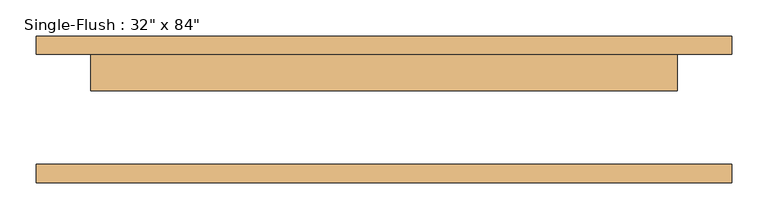
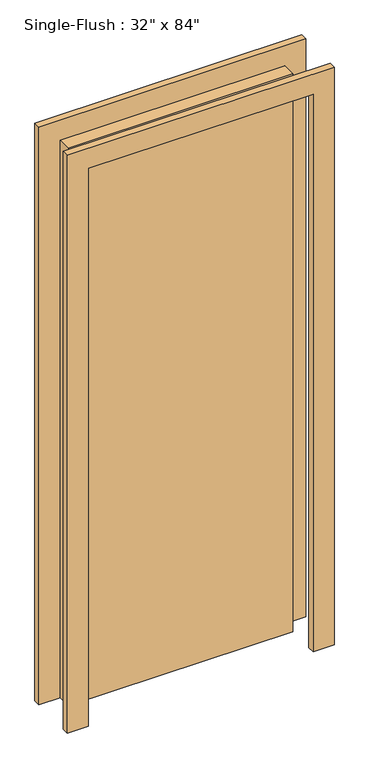
"""IFC4 building model written with IfcOpenShell, lengths in millimetres: door geometry."""

from ifc_helpers import new_model, si_unit, frame, origin, origin_with_axes, place, context, project, spatial, polyline, outline, extrude, source, transform, mapped, element, save


def door_377e7377(model_context):
    return source(origin(), model_context, "Body", "SweptSolid", [
        extrude(outline(polyline([(2209.8, -482.6), (0.0, -482.6), (0.0, -406.4), (2133.6, -406.4), (2133.6, 406.4), (0.0, 406.4), (0.0, 482.6), (2209.8, 482.6), (2209.8, -482.6)])), frame((0.0, 76.2, 0.0), z_axis=(0.0, 1.0, 0.0), x_axis=(0.0, 0.0, 1.0)), (0.0, 0.0, 1.0), 25.4),
        extrude(outline(polyline([(2209.8, 482.6), (2209.8, -482.6), (0.0, -482.6), (0.0, -406.4), (2133.6, -406.4), (2133.6, 406.4), (0.0, 406.4), (0.0, 482.6), (2209.8, 482.6)])), frame((0.0, -101.6, 0.0), z_axis=(0.0, 1.0, 0.0), x_axis=(0.0, 0.0, 1.0)), (0.0, 0.0, 1.0), 25.4),
        extrude(outline(polyline([(406.4, 25.4), (-406.4, 25.4), (-406.4, 76.2), (406.4, 76.2), (406.4, 25.4)])), origin_with_axes(), (0.0, 0.0, 1.0), 2133.6),
    ])


if __name__ == "__main__":
    model = new_model("IFC4")
    model_context = context("Model", 3, world=origin())
    ifc_project = project(units=[si_unit("LENGTHUNIT", "METRE", prefix="MILLI")], contexts=[model_context])
    site = spatial("IfcSite", under=ifc_project)
    building = spatial("IfcBuilding", under=site)
    placement = place(None, origin())
    door_shape = door_377e7377(model_context)
    element("IfcDoor", 1, ObjectType="Single-Flush : 32\" x 84\"", at=placement, inside=building, context=model_context, shape_type="MappedRepresentation", body=[
        mapped(door_shape, transform((0.0, 0.0, 0.0), x_axis=(1.0, 0.0, 0.0), y_axis=(0.0, 1.0, 0.0), z_axis=(0.0, 0.0, 1.0))),
    ])
    save(model, "model.ifc")

# Revit data of these elements
# Type "Single-Flush : 32\" x 84\""
#   Type Mark = "3"
#   Construction Type Id = "MDOOR"
#   Assembly Code = "C1020"
#   Analytic Construction = "Metal"
#   Thickness = 0' - 2"
#   Heat Transfer Coefficient (U) = 0.651978 BTU/(h·ft²·°F)
#   Height = 7' - 0"
#   Trim Projection Ext = 0' - 1"
#   Trim Projection Int = 0' - 1"
#   Trim Width = 0' - 3"
#   Width = 2' - 8"
#   Define Thermal Properties by = 1
#   Door Material = Door - Panel
#   Frame Material = Door - Frame
#   Visual Light Transmittance = 0
#   Solar Heat Gain Coefficient = 0
#   Function = (empty or 0)
#   Wall Closure = (empty or 0)
# Element 1 (IfcDoor, "Single-Flush : 32\" x 84\"")
#   Materials on its faces: "Door - Frame", "Door - Panel"
# Materials
#   "Door - Panel": class "Wood", colour RGB 210 159 95, transparency 0
#   "Door - Frame": colour RGB 118 70 51, transparency 0
